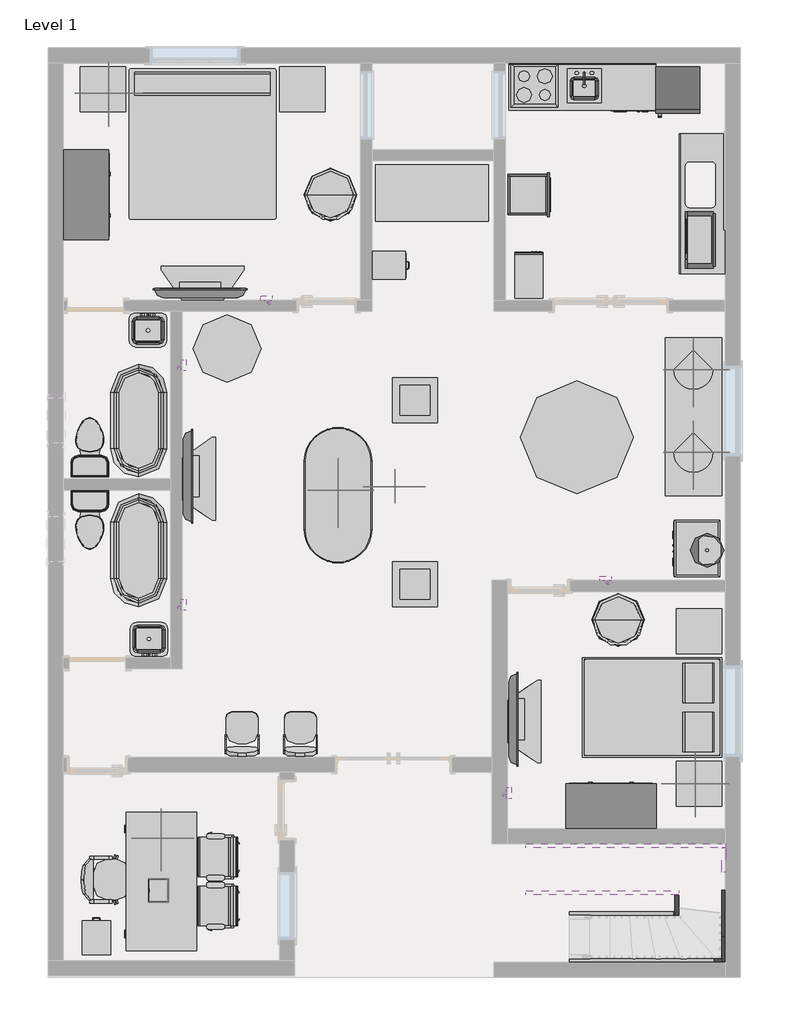
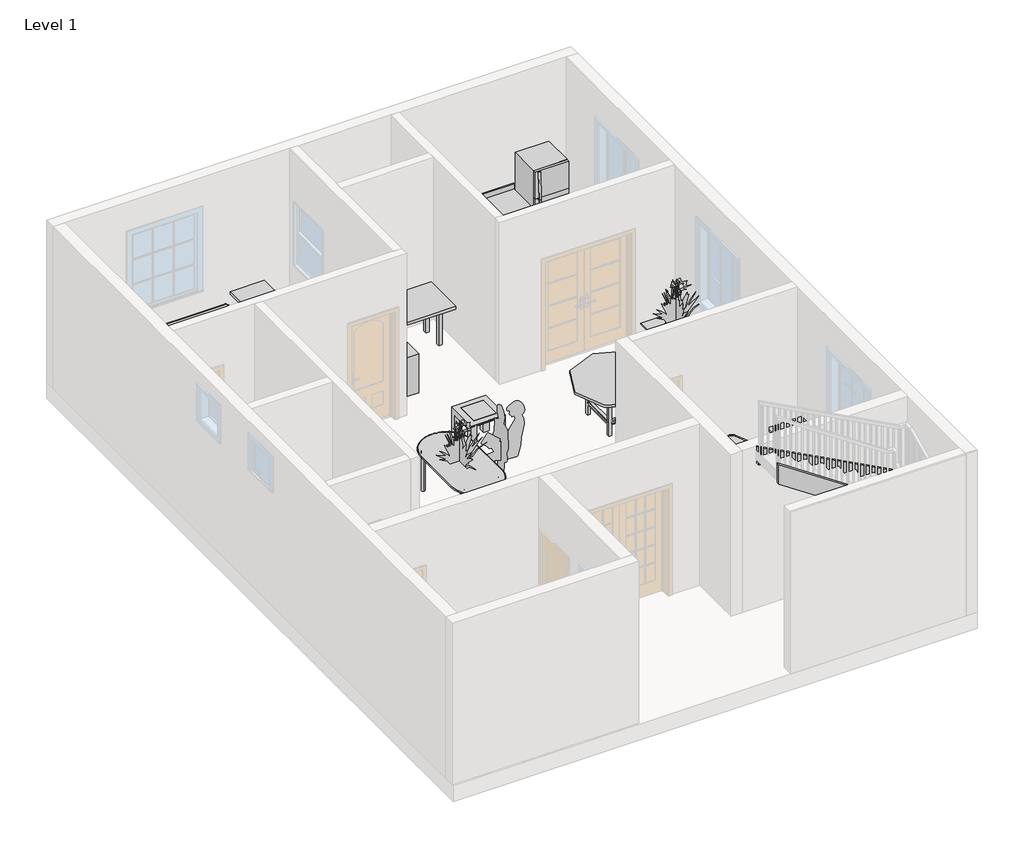
# One storey, part 3 of 3: 34 furniture elements, 14 proxies, 8 flow terminals, 8 members, 6 geographic elements.
"""IFC4 building model written with IfcOpenShell, lengths in millimetres."""

from ifc_helpers import new_model, si_unit, frame, origin, place, context, project, spatial, polyline, outline, extrude, transform, mapped, element, save
from components import entourage_4c8cfd20, proxy_db4bb64d, proxy_a6faaae8, proxy_45b28599, kitchenette_medium_kitchenette_medium_844211aa, proxy_8a8d5ab2, proxy_8b8c2dc4, rpc_female_69e001fa, rpc_picture_frame_rpc_picture_frame_c25e3fe9, proxy_c523a7b7, flow_terminal_871c2e40, flow_terminal_d49f872f, flow_terminal_62a433f7, toilet_domestic_3d_toilet_domestic_3d_f7549cf7, toilet_domestic_3d_toilet_domestic_3d_183bbd19, flow_terminal_b374fae2, furniture_338da5bd, furniture_c8abb964, furniture_1fc5af50, furniture_bb55ed6b, furniture_552c1472, chair_executive_chair_executive_8d69e98c, chair_task_arms_chair_task_arms_fa5a08ef, counter_top_w_sink_hole_0600mm_depth_1dfd4d8d, furniture_c6510c7c, furniture_2fc54265, furniture_9fa109b2, furniture_3d1d9cbc, furniture_fdf74506, tv_stand_tv_stand_6ce107e5, furniture_b5c51a22, furniture_92191dda, furniture_2c34a4f9, furniture_bbcc68ce, furniture_4bee3317, furniture_5bc9ed15, furniture_d900495b, furniture_a7e4c93f, rpc_plant_tropical_55f6ff97, rpc_plant_tropical_agave_1_5_93a2a214, rpc_plant_tropical_dagger_2_80c14bd7

model = new_model("IFC4")

# Units and contexts
model_context = context("Model", 3, world=origin())
ifc_project = project(units=[si_unit("LENGTHUNIT", "METRE", prefix="MILLI")], contexts=[model_context])

# Site, building, storey
site = spatial("IfcSite", under=ifc_project)
building = spatial("IfcBuilding", under=site)
storey = spatial("IfcBuildingStorey", under=building, Name="Level 1", Elevation=0.0)

# Proxies
placement = place(None, origin())
entourage_shape = entourage_4c8cfd20(model_context)
element("IfcBuildingElementProxy", 1, Name="Entourage", at=placement, inside=storey, context=model_context, shape_type="MappedRepresentation", body=[
    mapped(entourage_shape, transform((-5134.7041596, 1372.5606373, 762.0), x_axis=(0.0, -1.0, 0.0), y_axis=(1.0, 0.0, 0.0), z_axis=(0.0, 0.0, 1.0))),
])
proxy_shape = proxy_db4bb64d(model_context)
element("IfcBuildingElementProxy", 2, Name="15\" x 24\" x 34 1/2\"", ObjectType="15\" x 24\" x 34 1/2\"", at=placement, inside=storey, context=model_context, shape_type="MappedRepresentation", body=[
    mapped(proxy_shape, transform((99.0133089, 9939.509074, 0.0), x_axis=(-1.0, 0.0, 0.0), y_axis=(0.0, -1.0, 0.0), z_axis=(0.0, 0.0, 1.0))),
])
proxy_2_shape = proxy_a6faaae8(model_context)
element("IfcBuildingElementProxy", 3, Name="Cook Top-4 Unit2 : 22\" x 20\"", ObjectType="Cook Top-4 Unit2 : 22\" x 20\"", at=placement, inside=storey, context=model_context, shape_type="MappedRepresentation", body=[
    mapped(proxy_2_shape, transform((-92.8041596, 12238.4595092, 0.0), x_axis=(1.0, 0.0, 0.0), y_axis=(0.0, 1.0, 0.0), z_axis=(0.0, 0.0, 1.0))),
])
proxy_3_shape = proxy_45b28599(model_context)
element("IfcBuildingElementProxy", 4, Name="Dishwasher : 24\" x 24\" x 34\"", ObjectType="Dishwasher : 24\" x 24\" x 34\"", at=placement, inside=storey, context=model_context, shape_type="MappedRepresentation", body=[
    mapped(proxy_3_shape, transform((858.3783719, 11946.6099445, 0.0), x_axis=(1.0, 0.0, 0.0), y_axis=(0.0, 1.0, 0.0), z_axis=(0.0, 0.0, 1.0))),
])
kitchenette_medium_kitchenette_medium_shape = kitchenette_medium_kitchenette_medium_844211aa(model_context)
element("IfcBuildingElementProxy", 5, Name="Kitchenette - Medium : Kitchenette - Medium", ObjectType="Kitchenette - Medium : Kitchenette - Medium", at=placement, inside=storey, context=model_context, shape_type="MappedRepresentation", body=[
    mapped(kitchenette_medium_kitchenette_medium_shape, transform((231.3581355, 12543.2595092, 0.0), x_axis=(1.0, 0.0, 0.0), y_axis=(0.0, 1.0, 0.0), z_axis=(0.0, 0.0, 1.0))),
])
proxy_4_shape = proxy_8a8d5ab2(model_context)
element("IfcBuildingElementProxy", 6, Name="Microwave : 30\" x 16\" x 18\"", ObjectType="Microwave : 30\" x 16\" x 18\"", at=placement, inside=storey, context=model_context, shape_type="MappedRepresentation", body=[
    mapped(proxy_4_shape, transform((2501.0325962, 10655.9523866, 0.0), x_axis=(0.0, -1.0000000000000004, 0.0), y_axis=(1.0000000000000004, 0.0, 0.0), z_axis=(0.0, 0.0, 1.0))),
])
proxy_5_shape = proxy_8b8c2dc4(model_context)
element("IfcBuildingElementProxy", 7, Name="Oven Double-Built-in : 21 1/2\" x 39 1/4\" x 21\"", ObjectType="Oven Double-Built-in : 21 1/2\" x 39 1/4\" x 21\"", at=placement, inside=storey, context=model_context, shape_type="MappedRepresentation", body=[
    mapped(proxy_5_shape, transform((-40.6383007, 10800.4344366, 0.0), x_axis=(0.0, 1.0000000000000007, 0.0), y_axis=(-1.0000000000000007, 0.0, 0.0), z_axis=(0.0, 0.0, 1.0))),
])
rpc_female_shape = rpc_female_69e001fa(model_context)
element("IfcBuildingElementProxy", 8, Name="RPC Female", ObjectType="RPC Female", at=placement, inside=storey, context=model_context, shape_type="MappedRepresentation", body=[
    mapped(rpc_female_shape, transform((-2137.5041596, 6832.0104482, 0.0), x_axis=(0.0, -1.0000000000000004, 0.0), y_axis=(1.0000000000000004, 0.0, 0.0), z_axis=(0.0, 0.0, 1.0))),
])
rpc_picture_frame_rpc_picture_frame_shape = rpc_picture_frame_rpc_picture_frame_c25e3fe9(model_context)
element("IfcBuildingElementProxy", 9, Name="RPC Picture Frame : RPC Picture Frame", ObjectType="RPC Picture Frame : RPC Picture Frame", at=placement, inside=storey, context=model_context, shape_type="MappedRepresentation", body=[
    mapped(rpc_picture_frame_rpc_picture_frame_shape, transform((-3713.0036891, 9342.8595092, 1524.0), x_axis=(-1.0, 0.0, 0.0), y_axis=(0.0, -1.0, 0.0), z_axis=(0.0, 0.0, 1.0))),
])
element("IfcBuildingElementProxy", 10, Name="RPC Picture Frame : RPC Picture Frame", ObjectType="RPC Picture Frame : RPC Picture Frame", at=placement, inside=storey, context=model_context, shape_type="MappedRepresentation", body=[
    mapped(rpc_picture_frame_rpc_picture_frame_shape, transform((-4855.3041596, 8463.5402001, 1524.0), x_axis=(0.0, 1.0000000000000004, 0.0), y_axis=(-1.0000000000000004, 0.0, 0.0), z_axis=(0.0, 0.0, 1.0))),
])
element("IfcBuildingElementProxy", 11, Name="RPC Picture Frame : RPC Picture Frame", ObjectType="RPC Picture Frame : RPC Picture Frame", at=placement, inside=storey, context=model_context, shape_type="MappedRepresentation", body=[
    mapped(rpc_picture_frame_rpc_picture_frame_shape, transform((-4855.3041596, 5230.0441867, 1524.0), x_axis=(0.0, 1.0000000000000002, 0.0), y_axis=(-1.0000000000000002, 0.0, 0.0), z_axis=(0.0, 0.0, 1.0))),
])
element("IfcBuildingElementProxy", 12, Name="RPC Picture Frame : RPC Picture Frame", ObjectType="RPC Picture Frame : RPC Picture Frame", at=placement, inside=storey, context=model_context, shape_type="MappedRepresentation", body=[
    mapped(rpc_picture_frame_rpc_picture_frame_shape, transform((-461.1041596, 2689.3565223, 1524.0), x_axis=(0.0, 1.0000000000000009, 0.0), y_axis=(-1.0000000000000009, 0.0, 0.0), z_axis=(0.0, 0.0, 1.0))),
])
element("IfcBuildingElementProxy", 13, Name="RPC Picture Frame : RPC Picture Frame", ObjectType="RPC Picture Frame : RPC Picture Frame", at=placement, inside=storey, context=model_context, shape_type="MappedRepresentation", body=[
    mapped(rpc_picture_frame_rpc_picture_frame_shape, transform((869.3388904, 5558.2595092, 1524.0), x_axis=(-1.0, 0.0, 0.0), y_axis=(0.0, -1.0, 0.0), z_axis=(0.0, 0.0, 1.0))),
])
proxy_6_shape = proxy_c523a7b7(model_context)
element("IfcBuildingElementProxy", 14, Name="Refrigerator : 24\" x 25\" LH", ObjectType="Refrigerator : 24\" x 25\" LH", at=placement, inside=storey, context=model_context, shape_type="MappedRepresentation", body=[
    mapped(proxy_6_shape, transform((1843.9458404, 12192.8105378, 0.0), x_axis=(1.0, 0.0, 0.0), y_axis=(0.0, 1.0, 0.0), z_axis=(0.0, 0.0, 1.0))),
])

# Flow terminals
flow_terminal_shape = flow_terminal_871c2e40(model_context)
element("IfcFlowTerminal", 15, ObjectType="Sink Kitchen-Island : 18\" x 18\"", at=placement, inside=storey, context=model_context, shape_type="MappedRepresentation", body=[
    mapped(flow_terminal_shape, transform((564.6065998, 12236.1141081, -14.4), x_axis=(1.0, 0.0, 0.0), y_axis=(0.0, 1.0, 0.0), z_axis=(0.0, 0.0, 1.0))),
])
flow_terminal_2_shape = flow_terminal_d49f872f(model_context)
element("IfcFlowTerminal", 16, ObjectType="Sink Vanity-Round : 19\" x 19\"", at=placement, inside=storey, context=model_context, shape_type="MappedRepresentation", body=[
    mapped(flow_terminal_2_shape, transform((2324.0435785, 5868.0077687, 431.8), x_axis=(0.0, 1.0000000000000002, 0.0), y_axis=(-1.0000000000000002, 0.0, 0.0), z_axis=(0.0, 0.0, 1.0))),
])
flow_terminal_3_shape = flow_terminal_62a433f7(model_context)
element("IfcFlowTerminal", 17, ObjectType="Sink Vanity-Square : 20\" x 18\"", at=placement, inside=storey, context=model_context, shape_type="MappedRepresentation", body=[
    mapped(flow_terminal_3_shape, transform((-5328.1934002, 8984.9141081, 304.8), x_axis=(1.0, 0.0, 0.0), y_axis=(0.0, 1.0, 0.0), z_axis=(0.0, 0.0, 1.0))),
])
element("IfcFlowTerminal", 18, ObjectType="Sink Vanity-Square : 20\" x 18\"", at=placement, inside=storey, context=model_context, shape_type="MappedRepresentation", body=[
    mapped(flow_terminal_3_shape, transform((-5284.114919, 4716.0549104, 304.8), x_axis=(-1.0000000000000004, 0.0, 0.0), y_axis=(0.0, -1.0000000000000004, 0.0), z_axis=(0.0, 0.0, 1.0))),
])
toilet_domestic_3d_toilet_domestic_3d_shape = toilet_domestic_3d_toilet_domestic_3d_f7549cf7(model_context)
toilet_domestic_3d_toilet_domestic_3d_2_shape = toilet_domestic_3d_toilet_domestic_3d_183bbd19(model_context)
element("IfcFlowTerminal", 19, ObjectType="Toilet-Domestic-3D : Toilet-Domestic-3D", at=placement, inside=storey, context=model_context, shape_type="MappedRepresentation", body=[
    mapped(toilet_domestic_3d_toilet_domestic_3d_shape, transform((-6099.9041596, 6282.7634819, 0.0), x_axis=(1.0, 0.0, 0.0), y_axis=(0.0, 1.0, 0.0), z_axis=(0.0, 0.0, 1.0))),
    mapped(toilet_domestic_3d_toilet_domestic_3d_2_shape, transform((-6099.9041596, 6282.7634819, 0.0), x_axis=(1.0, 0.0, 0.0), y_axis=(0.0, 1.0, 0.0), z_axis=(0.0, 0.0, 1.0))),
])
element("IfcFlowTerminal", 20, ObjectType="Toilet-Domestic-3D : Toilet-Domestic-3D", at=placement, inside=storey, context=model_context, shape_type="MappedRepresentation", body=[
    mapped(toilet_domestic_3d_toilet_domestic_3d_shape, transform((-6099.9041596, 7449.9555366, 0.0), x_axis=(-1.0000000000000004, 0.0, 0.0), y_axis=(0.0, -1.0000000000000004, 0.0), z_axis=(0.0, 0.0, 1.0))),
    mapped(toilet_domestic_3d_toilet_domestic_3d_2_shape, transform((-6099.9041596, 7449.9555366, 0.0), x_axis=(-1.0000000000000004, 0.0, 0.0), y_axis=(0.0, -1.0000000000000004, 0.0), z_axis=(0.0, 0.0, 1.0))),
])
flow_terminal_4_shape = flow_terminal_b374fae2(model_context)
element("IfcFlowTerminal", 21, ObjectType="Tub-Free Standing-3D : 30\" x 60\"", at=placement, inside=storey, context=model_context, shape_type="MappedRepresentation", body=[
    mapped(flow_terminal_4_shape, transform((-5439.5041596, 5964.6595092, 0.0), x_axis=(1.0, 0.0, 0.0), y_axis=(0.0, 1.0, 0.0), z_axis=(0.0, 0.0, 1.0))),
])
element("IfcFlowTerminal", 22, ObjectType="Tub-Free Standing-3D : 30\" x 60\"", at=placement, inside=storey, context=model_context, shape_type="MappedRepresentation", body=[
    mapped(flow_terminal_4_shape, transform((-5439.5041596, 7717.2595092, 0.0), x_axis=(-1.0000000000000002, 0.0, 0.0), y_axis=(0.0, -1.0000000000000002, 0.0), z_axis=(0.0, 0.0, 1.0))),
])

# Furniture
furniture_shape = furniture_338da5bd(model_context)
element("IfcFurniture", 23, ObjectType="30\"", at=placement, inside=storey, context=model_context, shape_type="MappedRepresentation", body=[
    mapped(furniture_shape, transform((2409.0958404, 6008.7972142, 0.0), x_axis=(0.0, -1.0, 0.0), y_axis=(1.0, 0.0, 0.0), z_axis=(0.0, 0.0, 1.0))),
])
furniture_2_shape = furniture_c8abb964(model_context)
element("IfcFurniture", 24, ObjectType="Bed-Box : Double 53\" x 74\"", at=placement, inside=storey, context=model_context, shape_type="MappedRepresentation", body=[
    mapped(furniture_2_shape, transform((1729.1253486, 4182.9119683, 0.0), x_axis=(0.0, -0.9999999999999998, 0.0), y_axis=(0.9999999999999998, 0.0, 0.0), z_axis=(0.0, 0.0, 1.0))),
])
furniture_3_shape = furniture_1fc5af50(model_context)
element("IfcFurniture", 25, ObjectType="Bed-Standard.0001 : King 78\" x 80\"", at=placement, inside=storey, context=model_context, shape_type="MappedRepresentation", body=[
    mapped(furniture_3_shape, transform((-4847.3926842, 11496.6545912, 0.0), x_axis=(1.0, 0.0, 0.0), y_axis=(0.0, 1.0, 0.0), z_axis=(0.0, 0.0, 1.0))),
])
furniture_4_shape = furniture_bb55ed6b(model_context)
element("IfcFurniture", 26, ObjectType="Cabinet-File 2 Drawer : 15\" x 18\"", at=placement, inside=storey, context=model_context, shape_type="MappedRepresentation", body=[
    mapped(furniture_4_shape, transform((-2203.4384597, 9940.6559563, 0.0), x_axis=(0.0, 1.0000000000000002, 0.0), y_axis=(-1.0000000000000002, 0.0, 0.0), z_axis=(0.0, 0.0, 1.0))),
])
furniture_5_shape = furniture_552c1472(model_context)
element("IfcFurniture", 27, ObjectType="Cabinet-File 3 Drawer : 15\" x 18\"", at=placement, inside=storey, context=model_context, shape_type="MappedRepresentation", body=[
    mapped(furniture_5_shape, transform((-6138.9006066, 590.1252091, 0.0), x_axis=(-1.0000000000000002, 0.0, 0.0), y_axis=(0.0, -1.0000000000000002, 0.0), z_axis=(0.0, 0.0, 1.0))),
])
chair_executive_chair_executive_shape = chair_executive_chair_executive_8d69e98c(model_context)
element("IfcFurniture", 28, ObjectType="Chair-Executive : Chair-Executive", at=placement, inside=storey, context=model_context, shape_type="MappedRepresentation", body=[
    mapped(chair_executive_chair_executive_shape, transform((-5864.8500612, 1660.6503289, 0.0), x_axis=(0.0, -1.0000000000000004, 0.0), y_axis=(1.0000000000000004, 0.0, 0.0), z_axis=(0.0, 0.0, 1.0))),
])
chair_task_arms_chair_task_arms_shape = chair_task_arms_chair_task_arms_fa5a08ef(model_context)
element("IfcFurniture", 29, ObjectType="Chair-Task Arms : Chair-Task Arms", at=placement, inside=storey, context=model_context, shape_type="MappedRepresentation", body=[
    mapped(chair_task_arms_chair_task_arms_shape, transform((-4353.758258, 1683.4686896, 0.0), x_axis=(0.0, 1.0000000000000002, 0.0), y_axis=(-1.0000000000000002, 0.0, 0.0), z_axis=(0.0, 0.0, 1.0))),
])
element("IfcFurniture", 30, ObjectType="Chair-Task Arms : Chair-Task Arms", at=placement, inside=storey, context=model_context, shape_type="MappedRepresentation", body=[
    mapped(chair_task_arms_chair_task_arms_shape, transform((-4353.758258, 1023.0686896, 0.0), x_axis=(0.0, 1.0000000000000002, 0.0), y_axis=(-1.0000000000000002, 0.0, 0.0), z_axis=(0.0, 0.0, 1.0))),
])
counter_top_w_sink_hole_0600mm_depth_shape = counter_top_w_sink_hole_0600mm_depth_1dfd4d8d(model_context)
element("IfcFurniture", 31, ObjectType="Counter Top w Sink Hole : 0600mm Depth", at=placement, inside=storey, context=model_context, shape_type="MappedRepresentation", body=[
    mapped(counter_top_w_sink_hole_0600mm_depth_shape, transform((1860.6145904, 10898.9218043, 0.0), x_axis=(0.0, 1.0, 0.0), y_axis=(-1.0, 0.0, 0.0), z_axis=(0.0, 0.0, 1.0))),
])
furniture_6_shape = furniture_c6510c7c(model_context)
element("IfcFurniture", 32, ObjectType="Counter Top w Sink Hole : 24\" Depth", at=placement, inside=storey, context=model_context, shape_type="MappedRepresentation", body=[
    mapped(furniture_6_shape, transform((764.7581355, 12543.2595092, -14.4), x_axis=(1.0, 0.0, 0.0), y_axis=(0.0, 1.0, 0.0), z_axis=(0.0, 0.0, 1.0))),
])
furniture_7_shape = furniture_2fc54265(model_context)
element("IfcFurniture", 33, ObjectType="Desk : 72\" x 36\"", at=placement, inside=storey, context=model_context, shape_type="MappedRepresentation", body=[
    mapped(furniture_7_shape, transform((-4677.5041596, 579.8595092, 0.0), x_axis=(0.0, 1.0000000000000002, 0.0), y_axis=(-1.0000000000000002, 0.0, 0.0), z_axis=(0.0, 0.0, 1.0))),
])
furniture_8_shape = furniture_9fa109b2(model_context)
element("IfcFurniture", 34, ObjectType="Dresser : 48\" x 72\" x 24\"", at=placement, inside=storey, context=model_context, shape_type="MappedRepresentation", body=[
    mapped(furniture_8_shape, transform((-6513.8671137, 11034.4527691, 0.0), x_axis=(0.0, 1.0, 0.0), y_axis=(-1.0, 0.0, 0.0), z_axis=(0.0, 0.0, 1.0))),
])
element("IfcFurniture", 35, ObjectType="Dresser : 48\" x 72\" x 24\"", at=placement, inside=storey, context=model_context, shape_type="MappedRepresentation", body=[
    mapped(furniture_8_shape, transform((671.825327, 2147.0965551, 0.0), x_axis=(-1.0000000000000002, 0.0, 0.0), y_axis=(0.0, -1.0000000000000002, 0.0), z_axis=(0.0, 0.0, 1.0))),
])
furniture_9_shape = furniture_3d1d9cbc(model_context)
element("IfcFurniture", 36, ObjectType="Seating-Auditorium : 18\" x 24\" x 30\"", at=placement, inside=storey, context=model_context, shape_type="MappedRepresentation", body=[
    mapped(furniture_9_shape, transform((-3415.8320284, 3285.5840994, 0.0), x_axis=(1.0000000000000004, 0.0, 0.0), y_axis=(0.0, 1.0000000000000004, 0.0), z_axis=(0.0, 0.0, 1.0))),
])
element("IfcFurniture", 37, ObjectType="Seating-Auditorium : 18\" x 24\" x 30\"", at=placement, inside=storey, context=model_context, shape_type="MappedRepresentation", body=[
    mapped(furniture_9_shape, transform((-4203.2320284, 3285.5840994, 0.0), x_axis=(1.0, 0.0, 0.0), y_axis=(0.0, 1.0, 0.0), z_axis=(0.0, 0.0, 1.0))),
])
furniture_10_shape = furniture_fdf74506(model_context)
element("IfcFurniture", 38, ObjectType="TV - Flat Screen : 50\"", at=placement, inside=storey, context=model_context, shape_type="MappedRepresentation", body=[
    mapped(furniture_10_shape, transform((-382.5655359, 3689.7040234, 914.4), x_axis=(0.0, 1.0000000000000002, 0.0), y_axis=(-1.0000000000000002, 0.0, 0.0), z_axis=(0.0, 0.0, 1.0))),
])
element("IfcFurniture", 39, ObjectType="TV - Flat Screen : 50\"", at=placement, inside=storey, context=model_context, shape_type="MappedRepresentation", body=[
    mapped(furniture_10_shape, transform((-4612.3486737, 9431.3981329, 914.4), x_axis=(-1.0000000000000004, 0.0, 0.0), y_axis=(0.0, -1.0000000000000004, 0.0), z_axis=(0.0, 0.0, 1.0))),
])
element("IfcFurniture", 40, ObjectType="TV - Flat Screen : 50\"", at=placement, inside=storey, context=model_context, shape_type="MappedRepresentation", body=[
    mapped(furniture_10_shape, transform((-4776.7655359, 6966.3040234, 914.4), x_axis=(0.0, 1.0000000000000002, 0.0), y_axis=(-1.0000000000000002, 0.0, 0.0), z_axis=(0.0, 0.0, 1.0))),
])
tv_stand_tv_stand_shape = tv_stand_tv_stand_6ce107e5(model_context)
element("IfcFurniture", 41, ObjectType="TV Stand : TV Stand", at=placement, inside=storey, context=model_context, shape_type="MappedRepresentation", body=[
    mapped(tv_stand_tv_stand_shape, transform((-461.1041596, 3528.0715072, 0.0), x_axis=(0.0, 1.0000000000000002, 0.0), y_axis=(-1.0000000000000002, 0.0, 0.0), z_axis=(0.0, 0.0, 1.0))),
])
element("IfcFurniture", 42, ObjectType="TV Stand : TV Stand", at=placement, inside=storey, context=model_context, shape_type="MappedRepresentation", body=[
    mapped(tv_stand_tv_stand_shape, transform((-4450.7161575, 9342.8595092, 0.0), x_axis=(-1.0000000000000004, 0.0, 0.0), y_axis=(0.0, -1.0000000000000004, 0.0), z_axis=(0.0, 0.0, 1.0))),
])
element("IfcFurniture", 43, ObjectType="TV Stand : TV Stand", at=placement, inside=storey, context=model_context, shape_type="MappedRepresentation", body=[
    mapped(tv_stand_tv_stand_shape, transform((-4855.3041596, 6804.6715072, 0.0), x_axis=(0.0, 1.0000000000000004, 0.0), y_axis=(-1.0000000000000004, 0.0, 0.0), z_axis=(0.0, 0.0, 1.0))),
])
furniture_11_shape = furniture_b5c51a22(model_context)
element("IfcFurniture", 44, ObjectType="Table-Coffee : 24\" x 24\" x 24\"", at=placement, inside=storey, context=model_context, shape_type="MappedRepresentation", body=[
    mapped(furniture_11_shape, transform((-1723.9699263, 5412.2484314, 0.0), x_axis=(1.0, 0.0, 0.0), y_axis=(0.0, 1.0, 0.0), z_axis=(0.0, 0.0, 1.0))),
])
element("IfcFurniture", 45, ObjectType="Table-Coffee : 24\" x 24\" x 24\"", at=placement, inside=storey, context=model_context, shape_type="MappedRepresentation", body=[
    mapped(furniture_11_shape, transform((-1723.9699263, 7895.0984314, 0.0), x_axis=(1.0, 0.0, 0.0), y_axis=(0.0, 1.0, 0.0), z_axis=(0.0, 0.0, 1.0))),
])
furniture_12_shape = furniture_92191dda(model_context)
element("IfcFurniture", 46, ObjectType="Table-Dining : 30\" x 84\" x 22\"", at=placement, inside=storey, context=model_context, shape_type="MappedRepresentation", body=[
    mapped(furniture_12_shape, transform((2148.7069182, 7749.7937426, 0.0), x_axis=(0.0, 1.0000000000000002, 0.0), y_axis=(-1.0000000000000002, 0.0, 0.0), z_axis=(0.0, 0.0, 1.0))),
])
furniture_13_shape = furniture_2c34a4f9(model_context)
element("IfcFurniture", 47, ObjectType="Table-Dining Oval : 36\" x 72\"", at=placement, inside=storey, context=model_context, shape_type="MappedRepresentation", body=[
    mapped(furniture_13_shape, transform((-3105.2025202, 7109.4291814, 0.0), x_axis=(0.0, 1.0, 0.0), y_axis=(-1.0, 0.0, 0.0), z_axis=(0.0, 0.0, 1.0))),
])
furniture_14_shape = furniture_bbcc68ce(model_context)
element("IfcFurniture", 48, ObjectType="Table-Dining Round w Chairs : 36\" Diameter", at=placement, inside=storey, context=model_context, shape_type="MappedRepresentation", body=[
    mapped(furniture_14_shape, transform((375.0138732, 7673.5381978, 0.0), x_axis=(1.0, 0.0, 0.0), y_axis=(0.0, 1.0, 0.0), z_axis=(0.0, 0.0, 1.0))),
])
furniture_15_shape = furniture_4bee3317(model_context)
element("IfcFurniture", 49, ObjectType="Table-Ellipse : 72\" x 36\"", at=placement, inside=storey, context=model_context, shape_type="MappedRepresentation", body=[
    mapped(furniture_15_shape, transform((-4245.7041596, 8688.8095092, 0.0), x_axis=(1.0, 0.0, 0.0), y_axis=(0.0, 1.0, 0.0), z_axis=(0.0, 0.0, 1.0))),
])
furniture_16_shape = furniture_5bc9ed15(model_context)
element("IfcFurniture", 50, ObjectType="Table-Night Stand : 24\" x 24\" x 30\"", at=placement, inside=storey, context=model_context, shape_type="MappedRepresentation", body=[
    mapped(furniture_16_shape, transform((-6230.6377899, 11882.8595092, 0.0), x_axis=(1.0, 0.0, 0.0), y_axis=(0.0, 1.0, 0.0), z_axis=(0.0, 0.0, 1.0))),
])
element("IfcFurniture", 51, ObjectType="Table-Night Stand : 24\" x 24\" x 30\"", at=placement, inside=storey, context=model_context, shape_type="MappedRepresentation", body=[
    mapped(furniture_16_shape, transform((-3538.2377899, 11882.8595092, 0.0), x_axis=(1.0, 0.0, 0.0), y_axis=(0.0, 1.0, 0.0), z_axis=(0.0, 0.0, 1.0))),
])
element("IfcFurniture", 52, ObjectType="Table-Night Stand : 24\" x 24\" x 30\"", at=placement, inside=storey, context=model_context, shape_type="MappedRepresentation", body=[
    mapped(furniture_16_shape, transform((1821.1622101, 4567.6595092, 0.0), x_axis=(1.0, 0.0, 0.0), y_axis=(0.0, 1.0, 0.0), z_axis=(0.0, 0.0, 1.0))),
])
element("IfcFurniture", 53, ObjectType="Table-Night Stand : 24\" x 24\" x 30\"", at=placement, inside=storey, context=model_context, shape_type="MappedRepresentation", body=[
    mapped(furniture_16_shape, transform((1821.1622101, 2510.2595092, 0.0), x_axis=(1.0, 0.0, 0.0), y_axis=(0.0, 1.0, 0.0), z_axis=(0.0, 0.0, 1.0))),
])
furniture_17_shape = furniture_d900495b(model_context)
element("IfcFurniture", 54, ObjectType="Table-Rectangular : 72\" x 30\"", at=placement, inside=storey, context=model_context, shape_type="MappedRepresentation", body=[
    mapped(furniture_17_shape, transform((-1477.1041596, 10790.6595092, 0.0), x_axis=(1.0, 0.0, 0.0), y_axis=(0.0, 1.0, 0.0), z_axis=(0.0, 0.0, 1.0))),
])
furniture_18_shape = furniture_a7e4c93f(model_context)
element("IfcFurniture", 55, ObjectType="Table-Round : 36\" Diameter", at=placement, inside=storey, context=model_context, shape_type="MappedRepresentation", body=[
    mapped(furniture_18_shape, transform((-2848.7041596, 10765.2595092, 0.0), x_axis=(1.0, 0.0, 0.0), y_axis=(0.0, 1.0, 0.0), z_axis=(0.0, 0.0, 1.0))),
])
element("IfcFurniture", 56, ObjectType="Table-Round : 36\" Diameter", at=placement, inside=storey, context=model_context, shape_type="MappedRepresentation", body=[
    mapped(furniture_18_shape, transform((1037.4958404, 5024.8595092, 0.0), x_axis=(1.0, 0.0, 0.0), y_axis=(0.0, 1.0, 0.0), z_axis=(0.0, 0.0, 1.0))),
])

# Geographic elements
rpc_plant_tropical_shape = rpc_plant_tropical_55f6ff97(model_context)
element("IfcGeographicElement", 57, ObjectType="RPC Plant - Tropical", at=placement, inside=storey, context=model_context, shape_type="MappedRepresentation", body=[
    mapped(rpc_plant_tropical_shape, transform((-2747.1041596, 6777.4595092, 609.6), x_axis=(1.0, 0.0, 0.0), y_axis=(0.0, 1.0, 0.0), z_axis=(0.0, 0.0, 1.0))),
])
element("IfcGeographicElement", 58, ObjectType="RPC Plant - Tropical", at=placement, inside=storey, context=model_context, shape_type="MappedRepresentation", body=[
    mapped(rpc_plant_tropical_shape, transform((2053.4958404, 7285.4595092, 609.6), x_axis=(1.0, 0.0, 0.0), y_axis=(0.0, 1.0, 0.0), z_axis=(0.0, 0.0, 1.0))),
])
element("IfcGeographicElement", 59, ObjectType="RPC Plant - Tropical", at=placement, inside=storey, context=model_context, shape_type="MappedRepresentation", body=[
    mapped(rpc_plant_tropical_shape, transform((2053.4958404, 8403.0595092, 609.6), x_axis=(1.0, 0.0, 0.0), y_axis=(0.0, 1.0, 0.0), z_axis=(0.0, 0.0, 1.0))),
])
rpc_plant_tropical_agave_1_5_shape = rpc_plant_tropical_agave_1_5_93a2a214(model_context)
element("IfcGeographicElement", 60, ObjectType="RPC Plant - Tropical : Agave - 1.5'", at=placement, inside=storey, context=model_context, shape_type="MappedRepresentation", body=[
    mapped(rpc_plant_tropical_agave_1_5_shape, transform((-5845.9041596, 12136.8595092, 762.0), x_axis=(1.0, 0.0, 0.0), y_axis=(0.0, 1.0, 0.0), z_axis=(0.0, 0.0, 1.0))),
])
element("IfcGeographicElement", 61, ObjectType="RPC Plant - Tropical : Agave - 1.5'", at=placement, inside=storey, context=model_context, shape_type="MappedRepresentation", body=[
    mapped(rpc_plant_tropical_agave_1_5_shape, transform((2078.8958404, 2815.0595092, 762.0), x_axis=(1.0, 0.0, 0.0), y_axis=(0.0, 1.0, 0.0), z_axis=(0.0, 0.0, 1.0))),
])
rpc_plant_tropical_dagger_2_shape = rpc_plant_tropical_dagger_2_80c14bd7(model_context)
element("IfcGeographicElement", 62, ObjectType="RPC Plant - Tropical : Dagger - 2'", at=placement, inside=storey, context=model_context, shape_type="MappedRepresentation", body=[
    mapped(rpc_plant_tropical_dagger_2_shape, transform((-5134.7041596, 2078.4595092, 762.0), x_axis=(1.0, 0.0, 0.0), y_axis=(0.0, 1.0, 0.0), z_axis=(0.0, 0.0, 1.0))),
])

# Members
element("IfcMember", 63, ObjectType="Stringer - 2\" Width", at=placement, inside=storey, context=model_context, shape_type="SweptSolid", body=[
    extrude(outline(polyline([(193.214427, 376.3877765), (0.0, 376.3877765), (0.0, 630.5358859), (834.9174727, 1803.2275323), (1209.0769059, 1803.2275323), (193.214427, 376.3877765)])), frame((0.0, 1037.0595092, 0.0), z_axis=(0.0, 1.0, 0.0), x_axis=(0.0, 0.0, 1.0)), (0.0, 0.0, 1.0), 50.8),
])
element("IfcMember", 64, ObjectType="Stringer - 2\" Width", at=placement, inside=storey, context=model_context, shape_type="SweptSolid", body=[
    extrude(outline(polyline([(1037.0595092, 957.0117105), (1037.0595092, 1366.0008937), (1316.4595092, 1615.9823173), (1316.4595092, 1206.9931341), (1037.0595092, 957.0117105)])), frame((1803.2275323, 0.0, 0.0), z_axis=(1.0, 0.0, 0.0), x_axis=(0.0, 1.0, 0.0)), (0.0, 0.0, 1.0), 50.8),
])
element("IfcMember", 65, ObjectType="Stringer - 2\" Width", at=placement, inside=storey, context=model_context, shape_type="SweptSolid", body=[
    extrude(outline(polyline([(1362.6993804, 1854.0275323), (1730.0130308, 1854.0275323), (3115.8685207, -206.7168353), (2748.5548704, -206.7168353), (1362.6993804, 1854.0275323)])), frame((0.0, 1316.4595092, 0.0), z_axis=(0.0, 1.0, 0.0), x_axis=(0.0, 0.0, 1.0)), (0.0, 0.0, 1.0), 50.8),
])
element("IfcMember", 66, ObjectType="Stringer - 2\" Width", at=placement, inside=storey, context=model_context, shape_type="SweptSolid", body=[
    extrude(outline(polyline([(233.880429, 376.3877765), (0.0, 376.3877765), (0.0, 591.0647232), (913.240444, 2438.2275323), (1253.2575217, 2438.2275323), (233.880429, 376.3877765)])), frame((0.0, 402.0595092, 0.0), z_axis=(0.0, 1.0, 0.0), x_axis=(0.0, 0.0, 1.0)), (0.0, 0.0, 1.0), 50.8),
])
element("IfcMember", 67, ObjectType="Stringer - 2\" Width", at=placement, inside=storey, context=model_context, shape_type="SweptSolid", body=[
    extrude(outline(polyline([(2489.0275323, 402.0595092), (2438.2275323, 402.0595092), (2438.2275323, 747.5404846), (2489.0275323, 747.5404846), (2489.0275323, 402.0595092)])), frame((0.0, 0.0, 913.240444), z_axis=(0.0, 0.0, 1.0), x_axis=(1.0, 0.0, 0.0)), (0.0, 0.0, 1.0), 340.0170777),
])
element("IfcMember", 68, ObjectType="Stringer - 2\" Width", at=placement, inside=storey, context=model_context, shape_type="SweptSolid", body=[
    extrude(outline(polyline([(747.5404846, 913.240444), (747.5404846, 1253.2575217), (1615.7418959, 1651.0922227), (1615.7418959, 1311.075145), (747.5404846, 913.240444)])), frame((2438.2275323, 0.0, 0.0), z_axis=(1.0, 0.0, 0.0), x_axis=(0.0, 1.0, 0.0)), (0.0, 0.0, 1.0), 50.8),
])
element("IfcMember", 69, ObjectType="Stringer - 2\" Width", at=placement, inside=storey, context=model_context, shape_type="SweptSolid", body=[
    extrude(outline(polyline([(2489.0275323, 1615.7418959), (2438.2275323, 1615.7418959), (2438.2275323, 1951.4595092), (2489.0275323, 1951.4595092), (2489.0275323, 1615.7418959)])), frame((0.0, 0.0, 1313.2112997), z_axis=(0.0, 0.0, 1.0), x_axis=(1.0, 0.0, 0.0)), (0.0, 0.0, 1.0), 335.2763192),
])
element("IfcMember", 70, ObjectType="Stringer - 2\" Width", at=placement, inside=storey, context=model_context, shape_type="SweptSolid", body=[
    extrude(outline(polyline([(1343.6876189, 2489.0275323), (1621.4093099, 2489.0275323), (3058.3423615, -206.7168353), (2723.0660423, -206.7168353), (1343.6876189, 2381.0527281), (1343.6876189, 2489.0275323)])), frame((0.0, 1951.4595092, 0.0), z_axis=(0.0, 1.0, 0.0), x_axis=(0.0, 0.0, 1.0)), (0.0, 0.0, 1.0), 50.8),
])

save(model, "model.ifc")

# Revit data of these elements
# Type
#   built-in parameter 1005195 = "RPC-16-N04H-AQSP-D1N4-43SU-6GKQ-C3KU-1C"
#   Height = 0
# Type "15\" x 24\" x 34 1/2\""
#   Label = "T"
#   Assembly Code = "E1090400"
#   Depth = 2' - 0"
#   Height = 2' - 10 1/2"
#   Width = 1' - 3"
#   Panel Face Material = Plastic, Opaque Black
#   Trach Compact. Material = Steel, Paint Finish, Ivory, Matte
#   Default Elevation = 0
# Type "Cook Top-4 Unit2 : 22\" x 20\""
#   Depth = 1' - 8"
#   Width = 1' - 10"
#   Burner Material = Steel, Chrome Plated
#   Cooktop Material = Steel, Polished
#   Default Elevation = 0
#   Assembly Code = ""
# Type "Dishwasher : 24\" x 24\" x 34\""
#   Label = "DW"
#   Assembly Code = "E1090400"
#   Depth = 2' - 0"
#   Height = 2' - 10"
#   Width = 2' - 0"
#   Dishwasher Material = Steel, Paint Finish, Ivory, Glossy
#   Panel Face Material = Plastic, Opaque Black
#   Default Elevation = 0
# Type "Kitchenette - Medium : Kitchenette - Medium"
#   Assembly Code = "E1090400"
#   Counter Length = 6' - 6"
#   Cabinet Width = 4' - 6"
#   Cabinet Height = 2' - 10 1/2"
#   Cabinet Depth = 2' - 0"
#   Toe Depth = 0' - 3"
#   Toe Height = 0' - 3 1/2"
#   Cabinet Material = Cabinets
#   Door/Drawer Material = Cabinets
#   Handle Material = Cabinets - Handles
#   Default Elevation = 0
# Type "Microwave : 30\" x 16\" x 18\""
#   Assembly Code = "E1090400"
#   Depth = 1' - 4"
#   Height = 1' - 6"
#   Width = 2' - 6"
#   Microwave Material = Laminate, Ivory, Matte
#   Default Elevation = 0
# Type "Oven Double-Built-in : 21 1/2\" x 39 1/4\" x 21\""
#   Label = "OVEN"
#   Assembly Code = "E1090400"
#   Depth = 1' - 9"
#   Height = 3' - 3 1/4"
#   Width = 1' - 9 1/2"
#   Oven Material = Metal - Stainless Steel, Polished
#   Default Elevation = 0
# Type "RPC Female"
#   built-in parameter 1005195 = "RPC-8-FXA2-QQQ0-UGV2-6"
#   Height = 0
# Type "RPC Picture Frame : RPC Picture Frame"
#   built-in parameter 1005198 = "{2, 15},{39, RPC-16-8M5E-0H3T-F0AH-3U0K-JLQ7-G28B-AU},{1, 0},{1, 0},{2, 19},{1, 8},{5, Color},{1, 0},{1, 0},{3, 0.8},{3, 0.8},{3, 0.8},{1, 8},{7, BBoxMin},{1, 0},{1, 0},{1, 0},{1, 0},{1, 0},{1, 8},{7, BBoxMax},{1, 0},{1, 0},{1, 0},{1, 0},{1, 0},{2, 11},{9, RPCTypeId},{1, 0},{1, 0},{39, RPC-16-8M5E-0H3T-F0AH-3U0K-JLQ7-G28B-AU},{1, 6},{14, RPCPlantHeight},{1, 0},{1, 0},{5, 0.625},{2, 11},{7, keyword},{1, 0},{1, 0},{33, :RPCs:Office Clutter:Geometry:RPC},{2, 11},{8, category},{1, 0},{1, 0},{14, Office Clutter},{2, 11},{12, LocalizedUID},{1, 0},{1, 0},{13, Picture Frame},{2, 14},{6, Height},{1, 0},{1, 0},{5, 0.625},{1, 2},{16, Cast Reflections},{1, 0},{1, 0},{1, 0},{1, 2},{8, Portrait},{1, 0},{1, 0},{1, 1},{1, 2},{5, Stand},{1, 0},{1, 0},{1, 1},{2, 11},{10, RPCL_Frame},{1, 0},{1, 0},{5, Frame},{1, 4},{14, Frame Material},{1, 0},{1, 0},{1, 0},{2, 11},{12, RPCL_Picture},{1, 0},{1, 0},{7, Picture},{2, 11},{15, Picture Preview},{1, 0},{1, 0},{65, __RPC:/object data/textures/object/Photo/Photo0/textures/Portrait},{2, 11},{17, i_Picture Preview},{1, 0},{1, 0},{0, },{1, 2},{18, Use Custom Picture},{1, 0},{1, 0},{1, 0},{2, 11},{17, Picture File Name},{1, 0},{1, 0},{0, },{21, assetlibrary_base.fbx},{1, 5},"
#   built-in parameter 1005195 = "RPC-16-8M5E-0H3T-F0AH-3U0K-JLQ7-G28B-AU"
#   Height = 0
# Type "Refrigerator : 24\" x 25\" LH"
#   Label = "REF."
#   Assembly Code = "E1090400"
#   Depth = 2' - 0 3/4"
#   Handle = 0' - 1 1/2"
#   Height = 5' - 3 1/2"
#   Rear Clearance = 0' - 2"
#   Top Door Height = 1' - 8"
#   Width = 1' - 11 1/2"
#   Material = Steel, Paint Finish, Ivory, Glossy
#   Default Elevation = 0
# Type "Sink Kitchen-Island : 18\" x 18\""
#   Assembly Code = "D2010410"
#   Counter Height = 3' - 0"
#   Depth = 1' - 6"
#   Width = 1' - 6"
#   Faucet Material = Steel, Polished
#   Sink Material = Steel, Polished
#   Default Elevation = 0
# Type "Sink Vanity-Round : 19\" x 19\""
#   Assembly Code = "D2010400"
#   Top Of Counter = 2' - 7"
#   Basin Material = Porcelain, Linen
#   Faucet Material = Steel, Polished
#   Default Elevation = 0
# Type "Sink Vanity-Square : 20\" x 18\""
#   Assembly Code = "D2010400"
#   Counter Height = 2' - 7"
#   Depth = 1' - 6"
#   Width = 1' - 8"
#   Basin Material = Porcelain, Linen
#   Faucet Material = Steel, Polished
#   Default Elevation = 0
# Type "Toilet-Domestic-3D : Toilet-Domestic-3D"
#   Assembly Code = "D2010110"
#   Toilet - Bowl/Basin Material = Porcelain, Linen
#   Toilet - Seat Material = Laminate, Linen, Matte
#   Default Elevation = 0
# Type "Tub-Free Standing-3D : 30\" x 60\""
#   Assembly Code = "D2010110"
#   Height = 1' - 6"
#   Length = 5' - 0"
#   Width = 2' - 6"
#   Tub Material = Porcelain, Ivory
#   Default Elevation = 0
# Type "30\""
#   Assembly Code = "C1030410"
#   Depth = 2' - 0"
#   Height = 2' - 10 1/2"
#   Toe Depth = 0' - 3"
#   Toe Height = 0' - 3 1/2"
#   Width = 2' - 6"
#   Cabinet Material = none
#   Door/Drawer Material = none
#   Handle Material = Cabinets - Handles
#   Default Elevation = 0
# Type "Bed-Box : Double 53\" x 74\""
#   Assembly Code = "E2020200"
#   Length = 6' - 2"
#   Width = 4' - 5"
#   Frame Material = Birch
#   Mattress Material = Linen, White
#   Default Elevation = 0
# Type "Bed-Standard.0001 : King 78\" x 80\""
#   Assembly Code = "E2020200"
#   Length = 6' - 8"
#   Width = 6' - 6"
#   Leg Material = Steel, Chrome Plated
#   Mattress Material = Linen, White
#   Default Elevation = 0
# Type "Cabinet-File 2 Drawer : 15\" x 18\""
#   Assembly Code = "E2020200"
#   Depth = 1' - 6"
#   Height = 2' - 5"
#   Width = 1' - 3"
#   Cabinet Material = Steel, Paint Finish, Ivory, Glossy
#   Handle Material = Steel, Chrome Plated
#   Default Elevation = 0
# Type "Cabinet-File 3 Drawer : 15\" x 18\""
#   Assembly Code = "E2020200"
#   Depth = 1' - 6"
#   Height = 3' - 5"
#   Width = 1' - 3"
#   Cabinet Material = Steel, Paint Finish, Ivory, Glossy
#   Handle Material = Steel, Chrome Plated
#   Default Elevation = 0
# Type "Chair-Executive : Chair-Executive"
#   Assembly Code = "E2020200"
#   Base/Arms Material = Plastic, Opaque Black
#   Casters Material = Plastic, Opaque Black
#   Seat/Back Material = Textile - Slate Blue
#   Default Elevation = 0
# Type "Chair-Task Arms : Chair-Task Arms"
#   Assembly Code = "E2020200"
#   Base Material = Plastic, Opaque Black
#   Caster Material = Plastic, Opaque Black
#   Seat/Back Material = Textile - Slate Blue
#   Default Elevation = 0
# Type "Counter Top w Sink Hole : 0600mm Depth"
#   Assembly Code = "C1030400"
#   Counter Thickness = 0' - 1 9/16"
#   Depth = 2' - 0 19/32"
#   Height = 2' - 11 7/16"
#   Length [instance default] = 8' - 2 7/16"
#   Sink Location [instance default] = 3' - 11 1/4"
#   Sink Location To Wall [instance default] = 0' - 3 15/16"
#   Sink Opening Depth [instance default] = 1' - 2 7/8"
#   Sink Opening Width [instance default] = 1' - 11 1/8"
#   Counter Top Material = none
#   Default Elevation = 0
# Type "Counter Top w Sink Hole : 24\" Depth"
#   Assembly Code = "C1030400"
#   Counter Thickness = 0' - 1 1/2"
#   Depth = 2' - 1"
#   Height = 3' - 0"
#   Length [instance default] = 8' - 0"
#   Sink Location [instance default] = 2' - 0"
#   Sink Location To Wall [instance default] = 0' - 6"
#   Sink Opening Depth [instance default] = 1' - 3"
#   Sink Opening Width [instance default] = 2' - 3"
#   Counter Top Material = none
#   Default Elevation = 0
# Type "Desk : 72\" x 36\""
#   Assembly Code = "E2020200"
#   Depth = 3' - 0"
#   Height = 2' - 6"
#   Leg Height = 0' - 6"
#   Width = 6' - 0"
#   Body Material = Laminate, Ivory, Matte
#   Handle/Leg Material = Steel, Chrome Plated
#   Top Material = Cherry
#   Default Elevation = 0
# Type "Dresser : 48\" x 72\" x 24\""
#   Assembly Code = "E2020200"
#   Depth = 2' - 0"
#   Height = 6' - 0"
#   Width = 4' - 0"
#   Dresser Material = Laminate - Ivory, Glossy
#   Drawer Material = Laminate, Ivory, Matte
#   Knob Material = Cherry
#   Default Elevation = 0
# Type "Seating-Auditorium : 18\" x 24\" x 30\""
#   Assembly Code = "E2020200"
#   Seat Material = Linen, Beige
#   Frame Material = Steel, Paint Finish, Dark Gray, Matte
#   Default Elevation = 0
# Type "TV - Flat Screen : 50\""
#   SinAng = 0' - 0.0193"
#   L = 3' - 7.57782"
#   H = 2' - 0.51477"
#   Thickness = 0' - 4.33071"
#   Diagonal = 4' - 2"
#   CosAng = 0' - 0.03431"
#   Stand [instance default] = yes
#   Default Elevation = 0
# Type "TV Stand : TV Stand"
#   Depth = 1' - 6"
#   Width = 3' - 8"
#   Height = 1' - 7 1/2"
#   Finish = Melamine - Gray
#   Default Elevation = 0
# Type "Table-Coffee : 24\" x 24\" x 24\""
#   Assembly Code = "E2020200"
#   Height = 2' - 0"
#   Length = 2' - 0"
#   Width = 2' - 0"
#   Top Material = none
#   Frame Material = none
#   Default Elevation = 0
# Type "Table-Dining : 30\" x 84\" x 22\""
#   Assembly Code = "E2020200"
#   Height = 1' - 10"
#   Length = 7' - 0"
#   Width = 2' - 6"
#   Base Material = Steel, Chrome Plated
#   Top Material = Glass - Clear, Grey
#   Default Elevation = 0
# Type "Table-Dining Oval : 36\" x 72\""
#   Assembly Code = "E2020200"
#   Length = 6' - 0"
#   Width = 3' - 0"
#   Base Material = Steel, Chrome Plated
#   Top Material = Glass - Clear, Grey
#   Default Elevation = 0
#   Description = (empty or 0)
# Type "Table-Dining Round w Chairs : 36\" Diameter"
#   Assembly Code = "E2020200"
#   Radius = 2' - 6"
#   Diameter = 5' - 0"
#   Height = 2' - 6"
#   Chairs = 6
#   Base Material = Pine
#   Top Material = Laminate, Linen, Matte
#   Default Elevation = 0
# Type "Table-Ellipse : 72\" x 36\""
#   Assembly Code = "E2020200"
#   Half Width = 1' - 6"
#   Half Length = 1' - 6"
#   Height = 2' - 6"
#   Length = 3' - 0"
#   Width = 3' - 0"
#   Base Material = Birch
#   Top Material = Laminate - Black
#   Default Elevation = 0
# Type "Table-Night Stand : 24\" x 24\" x 30\""
#   Assembly Code = "E2020200"
#   Depth = 2' - 0"
#   Height = 2' - 6"
#   Width = 2' - 0"
#   Base Material = Birch
#   Top Material = Laminate, Ivory, Matte
#   Default Elevation = 0
# Type "Table-Rectangular : 72\" x 30\""
#   Assembly Code = "E2020200"
#   Height = 2' - 6"
#   Length = 5' - 0"
#   Width = 2' - 6"
#   Base Material = Birch
#   Top Material = Birch
#   Default Elevation = 0
# Type "Table-Round : 36\" Diameter"
#   Assembly Code = "E2020200"
#   Base Radius = 0' - 10"
#   Height = 2' - 6"
#   Radius = 1' - 2"
#   Base Material = Steel, Chrome Plated
#   Top Material = Birch
#   Default Elevation = 0
# Type "RPC Plant - Tropical"
#   built-in parameter 1005198 = "{2, 15},{39, RPC-16-FWM5-GM7X-C67P-4000-ST1L-LVER-AU},{1, 0},{1, 0},{2, 13},{1, 8},{5, Color},{1, 0},{1, 0},{3, 0.8},{3, 0.8},{3, 0.8},{1, 8},{7, BBoxMin},{1, 0},{1, 0},{1, 0},{1, 0},{1, 0},{1, 8},{7, BBoxMax},{1, 0},{1, 0},{1, 0},{1, 0},{1, 0},{2, 11},{9, RPCTypeId},{1, 0},{1, 0},{39, RPC-16-FWM5-GM7X-C67P-4000-ST1L-LVER-AU},{1, 6},{14, RPCPlantHeight},{1, 0},{1, 0},{1, 3},{2, 11},{7, keyword},{1, 0},{1, 0},{35, :RPCs:Shrubs [General]:Geometry:RPC},{2, 11},{8, category},{1, 0},{1, 0},{16, Shrubs [General]},{2, 11},{12, LocalizedUID},{1, 0},{1, 0},{10, Crane Lily},{2, 14},{6, Height},{1, 0},{1, 0},{1, 3},{1, 2},{16, Cast Reflections},{1, 0},{1, 0},{1, 0},{1, 2},{12, Cast Shadows},{1, 0},{1, 0},{1, 1},{1, 2},{9, Lock View},{1, 0},{1, 0},{1, 0},{1, 4},{5, ViewC},{1, 0},{1, 0},{1, 0},{21, assetlibrary_base.fbx},{1, 5},"
#   built-in parameter 1005195 = "RPC-16-FWM5-GM7X-C67P-4000-ST1L-LVER-AU"
#   Assembly Code = "G2050500"
#   Height = 3' - 0"
#   Default Elevation = 0
# Type "RPC Plant - Tropical : Agave - 1.5'"
#   built-in parameter 1005198 = "{2, 15},{39, RPC-16-G1GJ-63FX-7K5P-N000-ST1L-LVER-AU},{1, 0},{1, 0},{2, 13},{1, 8},{5, Color},{1, 0},{1, 0},{3, 0.8},{3, 0.8},{3, 0.8},{1, 8},{7, BBoxMin},{1, 0},{1, 0},{1, 0},{1, 0},{1, 0},{1, 8},{7, BBoxMax},{1, 0},{1, 0},{1, 0},{1, 0},{1, 0},{2, 11},{9, RPCTypeId},{1, 0},{1, 0},{39, RPC-16-G1GJ-63FX-7K5P-N000-ST1L-LVER-AU},{1, 6},{14, RPCPlantHeight},{1, 0},{1, 0},{3, 1.5},{2, 11},{7, keyword},{1, 0},{1, 0},{35, :RPCs:Plants [General]:Geometry:RPC},{2, 11},{8, category},{1, 0},{1, 0},{16, Plants [General]},{2, 11},{12, LocalizedUID},{1, 0},{1, 0},{5, Agave},{2, 14},{6, Height},{1, 0},{1, 0},{3, 1.5},{1, 2},{16, Cast Reflections},{1, 0},{1, 0},{1, 0},{1, 2},{12, Cast Shadows},{1, 0},{1, 0},{1, 1},{1, 2},{9, Lock View},{1, 0},{1, 0},{1, 0},{1, 4},{5, ViewC},{1, 0},{1, 0},{1, 0},{21, assetlibrary_base.fbx},{1, 5},"
#   built-in parameter 1005195 = "RPC-16-G1GJ-63FX-7K5P-N000-ST1L-LVER-AU"
#   Type Comments = "Agave"
#   Assembly Code = "G2050500"
#   Height = 1' - 6"
#   Default Elevation = 0
# Type "RPC Plant - Tropical : Dagger - 2'"
#   built-in parameter 1005198 = "{2, 15},{39, RPC-16-G3A7-NEG0-UH6H-J000-ST1L-LVER-AU},{1, 0},{1, 0},{2, 13},{1, 8},{5, Color},{1, 0},{1, 0},{3, 0.8},{3, 0.8},{3, 0.8},{1, 8},{7, BBoxMin},{1, 0},{1, 0},{1, 0},{1, 0},{1, 0},{1, 8},{7, BBoxMax},{1, 0},{1, 0},{1, 0},{1, 0},{1, 0},{2, 11},{9, RPCTypeId},{1, 0},{1, 0},{39, RPC-16-G3A7-NEG0-UH6H-J000-ST1L-LVER-AU},{1, 6},{14, RPCPlantHeight},{1, 0},{1, 0},{1, 2},{2, 11},{7, keyword},{1, 0},{1, 0},{35, :RPCs:Plants [General]:Geometry:RPC},{2, 11},{8, category},{1, 0},{1, 0},{16, Plants [General]},{2, 11},{12, LocalizedUID},{1, 0},{1, 0},{6, Dagger},{2, 14},{6, Height},{1, 0},{1, 0},{1, 2},{1, 2},{16, Cast Reflections},{1, 0},{1, 0},{1, 0},{1, 2},{12, Cast Shadows},{1, 0},{1, 0},{1, 1},{1, 2},{9, Lock View},{1, 0},{1, 0},{1, 0},{1, 4},{5, ViewC},{1, 0},{1, 0},{1, 0},{21, assetlibrary_base.fbx},{1, 5},"
#   built-in parameter 1005195 = "RPC-16-G3A7-NEG0-UH6H-J000-ST1L-LVER-AU"
#   Type Comments = "Dagger"
#   Assembly Code = "G2050500"
#   Height = 2' - 0"
#   Default Elevation = 0
# Element 1 (IfcBuildingElementProxy)
#   Phase Created = New Construction
# Element 2 (IfcBuildingElementProxy, "15\" x 24\" x 34 1/2\"")
#   Phase Created = New Construction
#   Materials on its faces: "Steel, Paint Finish, Ivory, Matte", "Plastic, Opaque Black"
# Element 3 (IfcBuildingElementProxy, "Cook Top-4 Unit2 : 22\" x 20\"")
#   Phase Created = New Construction
#   Materials on its faces: "Steel, Chrome Plated", "Steel, Polished"
# Element 4 (IfcBuildingElementProxy, "Dishwasher : 24\" x 24\" x 34\"")
#   Phase Created = New Construction
#   Materials on its faces: "Steel, Paint Finish, Ivory, Glossy", "Plastic, Opaque Black"
# Element 5 (IfcBuildingElementProxy, "Kitchenette - Medium : Kitchenette - Medium")
#   Phase Created = New Construction
#   Materials on its faces: "Cabinets", "Cabinets - Handles"
# Element 6 (IfcBuildingElementProxy, "Microwave : 30\" x 16\" x 18\"")
#   Phase Created = New Construction
#   Materials on its faces: "Laminate, Ivory, Matte", "Glass"
# Element 7 (IfcBuildingElementProxy, "Oven Double-Built-in : 21 1/2\" x 39 1/4\" x 21\"")
#   Phase Created = New Construction
#   Materials on its faces: "Steel", "Metal - Stainless Steel, Polished", "Glass"
# Element 8 (IfcBuildingElementProxy, "RPC Female")
#   Phase Created = New Construction
# Elements 9, 10, 11, 12, 13 (IfcBuildingElementProxy, "RPC Picture Frame : RPC Picture Frame")
#   Phase Created = New Construction
# Element 14 (IfcBuildingElementProxy, "Refrigerator : 24\" x 25\" LH")
#   Phase Created = New Construction
#   Materials on its faces: "Steel, Paint Finish, Ivory, Glossy", "Steel, Chrome Plated"
# Element 15 (IfcFlowTerminal, "Sink Kitchen-Island : 18\" x 18\"")
#   Mark = "8"
#   Phase Created = New Construction
#   Materials on its faces: "Steel, Polished"
# Element 16 (IfcFlowTerminal, "Sink Vanity-Round : 19\" x 19\"")
#   Mark = "7"
#   Phase Created = New Construction
#   Materials on its faces: "Porcelain, Linen", "Steel, Polished"
# Element 17 (IfcFlowTerminal, "Sink Vanity-Square : 20\" x 18\"")
#   Mark = "5"
#   Phase Created = New Construction
#   Materials on its faces: "Porcelain, Linen", "Steel, Polished"
# Element 18 (IfcFlowTerminal, "Sink Vanity-Square : 20\" x 18\"")
#   Mark = "6"
#   Phase Created = New Construction
#   Materials on its faces: "Porcelain, Linen", "Steel, Polished"
# Element 19 (IfcFlowTerminal, "Toilet-Domestic-3D : Toilet-Domestic-3D")
#   Mark = "1"
#   Phase Created = New Construction
#   Materials on its faces: "Porcelain, Linen", "Laminate, Linen, Matte"
# Element 20 (IfcFlowTerminal, "Toilet-Domestic-3D : Toilet-Domestic-3D")
#   Mark = "2"
#   Phase Created = New Construction
#   Materials on its faces: "Porcelain, Linen", "Laminate, Linen, Matte"
# Element 21 (IfcFlowTerminal, "Tub-Free Standing-3D : 30\" x 60\"")
#   Mark = "3"
#   Phase Created = New Construction
#   Materials on its faces: "Porcelain, Ivory"
# Element 22 (IfcFlowTerminal, "Tub-Free Standing-3D : 30\" x 60\"")
#   Mark = "4"
#   Phase Created = New Construction
#   Materials on its faces: "Porcelain, Ivory"
# Element 23 (IfcFurniture, "30\"")
#   Phase Created = New Construction
#   Materials on its faces: "Cabinets", "Cabinets - Handles"
# Element 24 (IfcFurniture, "Bed-Box : Double 53\" x 74\"")
#   Phase Created = New Construction
#   Materials on its faces: "Birch", "Linen, White"
# Element 25 (IfcFurniture, "Bed-Standard.0001 : King 78\" x 80\"")
#   Phase Created = New Construction
#   Materials on its faces: "Linen, White", "Steel, Chrome Plated"
# Element 26 (IfcFurniture, "Cabinet-File 2 Drawer : 15\" x 18\"")
#   Phase Created = New Construction
#   Materials on its faces: "Steel, Chrome Plated", "Steel, Paint Finish, Ivory, Glossy"
# Element 27 (IfcFurniture, "Cabinet-File 3 Drawer : 15\" x 18\"")
#   Phase Created = New Construction
#   Materials on its faces: "Steel, Chrome Plated", "Steel, Paint Finish, Ivory, Glossy"
# Element 28 (IfcFurniture, "Chair-Executive : Chair-Executive")
#   Phase Created = New Construction
#   Materials on its faces: "Plastic, Opaque Black", "Textile - Slate Blue"
# Elements 29, 30 (IfcFurniture, "Chair-Task Arms : Chair-Task Arms")
#   Phase Created = New Construction
#   Materials on its faces: "Plastic, Opaque Black", "Textile - Slate Blue"
# Element 31 (IfcFurniture, "Counter Top w Sink Hole : 0600mm Depth")
#   Sink Opening Width = 1' - 11 1/8"
#   Sink Opening Depth = 1' - 2 7/8"
#   Sink Location To Wall = 0' - 3 15/16"
#   Sink Location = 3' - 11 1/4"
#   Length = 6' - 2 7/16"
#   Phase Created = New Construction
#   Materials on its faces: "Counter Top"
# Element 32 (IfcFurniture, "Counter Top w Sink Hole : 24\" Depth")
#   Sink Opening Depth = 1' - 2"
#   Sink Location To Wall = 0' - 6"
#   Length = 6' - 6"
#   Sink Location = 3' - 4"
#   Sink Opening Width = 1' - 4"
#   Phase Created = New Construction
#   Materials on its faces: "Counter Top"
# Element 33 (IfcFurniture, "Desk : 72\" x 36\"")
#   Phase Created = New Construction
#   Materials on its faces: "Steel, Chrome Plated", "Laminate, Ivory, Matte", "Cherry"
# Elements 34, 35 (IfcFurniture, "Dresser : 48\" x 72\" x 24\"")
#   Phase Created = New Construction
#   Materials on its faces: "Laminate, Ivory, Matte", "Cherry", "Laminate - Ivory, Glossy"
# Elements 36, 37 (IfcFurniture, "Seating-Auditorium : 18\" x 24\" x 30\"")
#   Phase Created = New Construction
#   Materials on its faces: "Steel, Paint Finish, Dark Gray, Matte", "Linen, Beige"
# Elements 38, 39, 40 (IfcFurniture, "TV - Flat Screen : 50\"")
#   Stand = yes
#   Phase Created = New Construction
#   Materials on its faces: "TV - Black", "TV - Glass", "TV - Screen"
# Elements 41, 42, 43 (IfcFurniture, "TV Stand : TV Stand")
#   Phase Created = New Construction
#   Materials on its faces: "Melamine - Gray", "Glass - Shelves"
# Elements 44, 45 (IfcFurniture, "Table-Coffee : 24\" x 24\" x 24\"")
#   Phase Created = New Construction
#   Materials on its faces: "Glass - Clear, Grey"
# Element 46 (IfcFurniture, "Table-Dining : 30\" x 84\" x 22\"")
#   Phase Created = New Construction
#   Materials on its faces: "Steel, Chrome Plated", "Glass - Clear, Grey"
# Element 47 (IfcFurniture, "Table-Dining Oval : 36\" x 72\"")
#   Phase Created = New Construction
#   Materials on its faces: "Steel, Chrome Plated", "Glass - Clear, Grey"
# Element 48 (IfcFurniture, "Table-Dining Round w Chairs : 36\" Diameter")
#   Phase Created = New Construction
#   Materials on its faces: "Pine", "Laminate, Linen, Matte"
# Element 49 (IfcFurniture, "Table-Ellipse : 72\" x 36\"")
#   Phase Created = New Construction
#   Materials on its faces: "Birch", "Laminate - Black"
# Elements 50, 51, 52, 53 (IfcFurniture, "Table-Night Stand : 24\" x 24\" x 30\"")
#   Phase Created = New Construction
#   Materials on its faces: "Birch", "Laminate, Ivory, Matte"
# Element 54 (IfcFurniture, "Table-Rectangular : 72\" x 30\"")
#   Phase Created = New Construction
#   Materials on its faces: "Birch"
# Elements 55, 56 (IfcFurniture, "Table-Round : 36\" Diameter")
#   Phase Created = New Construction
#   Materials on its faces: "Steel, Chrome Plated", "Birch"
# Elements 57, 58, 59 (IfcGeographicElement, "RPC Plant - Tropical")
#   Phase Created = New Construction
# Elements 60, 61 (IfcGeographicElement, "RPC Plant - Tropical : Agave - 1.5'")
#   Phase Created = New Construction
# Element 62 (IfcGeographicElement, "RPC Plant - Tropical : Dagger - 2'")
#   Phase Created = New Construction
# Elements 63, 64, 65, 66, 67, 68, 69, 70 (IfcMember, "Stringer - 2\" Width")
#   Phase Created = New Construction
# Materials
#   "Plastic, Opaque Black": class "Plastic", colour RGB 0 0 0, transparency 0, Description = "Plastic, generic, opaque black", Cost = 0
#   "Steel, Paint Finish, Ivory, Matte": class "Metal", colour RGB 247 247 239, transparency 0, Description = "Steel, paint finish, ivory, matte", Cost = 0
#   "Steel, Chrome Plated": class "Metal", colour RGB 17 17 17, transparency 0, Description = "Chromiuim plated steel", Cost = 0
#   "Steel, Polished": class "Metal", colour RGB 57 57 57, transparency 0, Description = "Polished steel", Cost = 0
#   "Steel, Paint Finish, Ivory, Glossy": class "Metal", colour RGB 247 247 239, transparency 0, Description = "Steel, paint finish, ivory, glossy", Cost = 0
#   "Cabinets": colour RGB 249 249 249, transparency 0
#   "Cabinets - Handles": class "Metal", colour RGB 57 57 57, transparency 0
#   "Laminate, Ivory, Matte": class "Plastic", colour RGB 247 247 239, transparency 0, Description = "Plastic Laminate - Ivory, Matte", Cost = 0
#   "Metal - Stainless Steel, Polished": class "Metal", colour RGB 216 216 216, transparency 0
#   "Porcelain, Linen": class "Ceramic", colour RGB 249 239 230, transparency 0, Description = "Porcelain, linen", Cost = 0
#   "Laminate, Linen, Matte": class "Plastic", colour RGB 249 239 230, transparency 0, Description = "Plastic Laminate - Linen, Matte", Cost = 0
#   "Porcelain, Ivory": class "Ceramic", colour RGB 247 247 239, transparency 0, Description = "Porcelain, ivory", Cost = 0
#   "Birch": class "Wood", colour RGB 224 178 126, transparency 0, Description = "Betula Alleghaniensis", Cost = 0
#   "Linen, White": class "Textile", colour RGB 247 247 239, transparency 0, Description = "Linen, white", Cost = 0
#   "Textile - Slate Blue": class "Fabric", colour RGB 98 102 118, transparency 0
#   "Cherry": class "Wood", colour RGB 226 177 128, transparency 0, Description = "Prunus Serotina", Cost = 0
#   "Laminate - Ivory, Glossy": colour RGB 247 247 239, transparency 0
#   "Linen, Beige": class "Textile", colour RGB 249 239 230, transparency 0, Description = "Linen, beige", Cost = 0
#   "Steel, Paint Finish, Dark Gray, Matte": class "Metal", colour RGB 98 98 98, transparency 0, Description = "Steel, paint finish, dark gray, matte", Cost = 0
#   "Melamine - Gray": class "Wood", colour RGB 49 49 49, transparency 0
#   "Glass - Clear, Grey": class "Glass", colour RGB 252 255 255, transparency 0.64
#   "Pine": class "Wood", colour RGB 223 192 134, transparency 0, Description = "Pinus Echinata", Cost = 0
#   "Laminate - Black": colour RGB 0 0 0, transparency 0
#   "Glass": class "Glass", colour RGB 0 128 192, transparency 0.75, Description = "Soda Lime Glass", Cost = 0
#   "Steel": class "Metal", colour RGB 247 247 247, transparency 0, Description = "Steel, mill finish", Cost = 0
#   "Counter Top": class "Wood", colour RGB 226 177 128, transparency 0
#   "TV - Black": colour RGB 49 49 49, transparency 0
#   "TV - Glass": colour RGB 157 157 157, transparency 0.9
#   "TV - Screen": colour RGB 0 0 0, transparency 0
#   "Glass - Shelves": class "Glass", colour RGB 167 167 167, transparency 0.9
